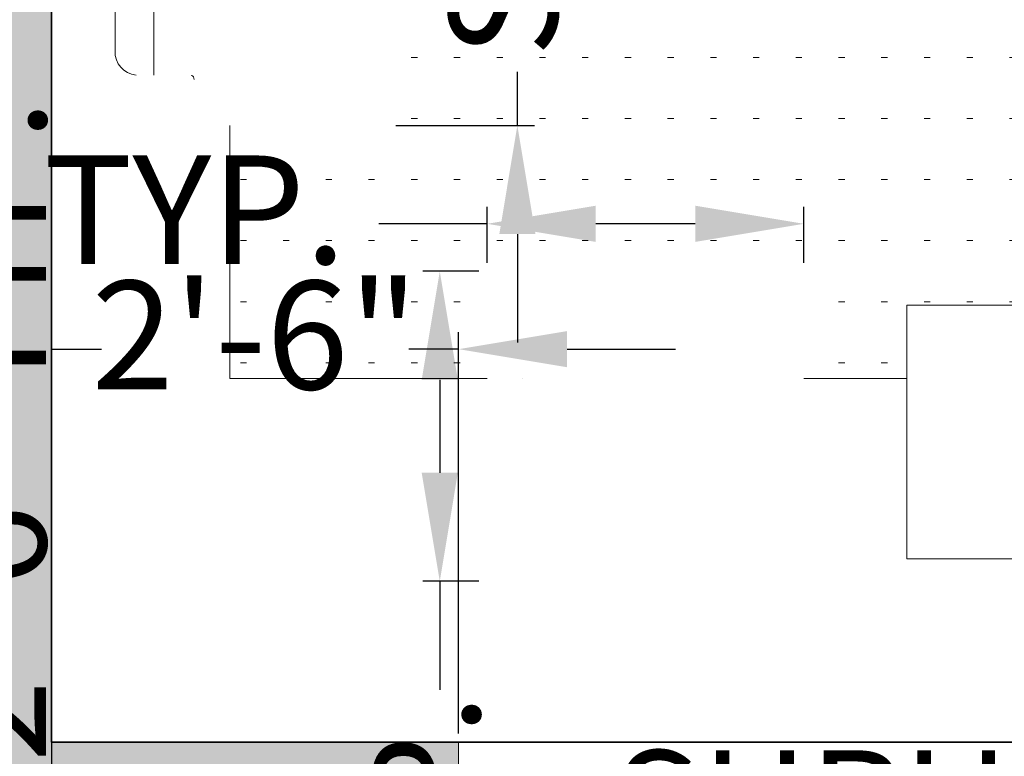
# Model space of a CAD drawing. Units: inches. Extents: x 2408 to 5087, y 2429 to 5085.
# Tile 4 of 12: x 2491 to 2564, y 2622 to 2676. Entities that reach past the tile are written whole.
import ezdxf

# ---------------------------------------------------------------- set-up
doc = ezdxf.new("R2010")
doc.units = ezdxf.units.IN
for name, color, linetype, lineweight in [('A-ANNO-DIMS', 2, 'Continuous', 18), ('A-FLOR-PATT', 8, 'Continuous', 13), ('A-FURN', 72, 'Continuous', 18), ('A-GLAZ', 4, 'Continuous', 18), ('A-WALL', 7, 'Continuous', 35), ('A-WALL-PATT', 252, 'Continuous', 13)]:
    doc.layers.add(name, color=color, linetype=linetype, lineweight=lineweight)
doc.styles.get("Standard").update_dxf_attribs({"font": 'arial.ttf'})
doc.dimstyles.new('ISO-25', dxfattribs={"dimtxt": 8, "dimasz": 8, "dimexe": 1.25, "dimexo": 0.625, "dimtad": 0, "dimdec": 1, "dimlunit": 4, "dimtxsty": 'Standard', "dimcen": 2.5, "dimadec": 0, "dimazin": 0, "dimtfac": 1, "dimtdec": 1, "dimtmove": 0, "dimatfit": 3, "dimfxl": 1, "dimarcsym": 0})

# ---------------------------------------------------------------- blocks, each defined once
blk = doc.blocks.new('Clinicians and patient chairs 9_dwgmodels.com')
at = {"color": 0}
for points in [[(-907.9, 0, 0, 0, 0), (-959.6, -11.1, 4.62, 4.62, 0)], [(907.9, 0, 0, 0, 0), (-907.9, 0, 4.62, 4.62, 0)], [(959.6, -11.1, 0, 0, 0), (907.9, 0, 4.62, 4.62, 0)], [(-959.6, -11.1, 0, 0, 0), (-994.7, -35.9, 4.62, 4.62, 0)], [(994.7, -35.9, 0, 0, 0), (959.6, -11.1, 4.62, 4.62, 0)], [(-994.7, -35.9, 0, 0, 0), (-1015.6, -68.3, 4.62, 4.62, 0)], [(1015.6, -68.3, 0, 0, 0), (994.7, -35.9, 4.62, 4.62, 0)], [(-1015.6, -68.3, 0, 0, 0), (-1025.5, -106.3, 4.62, 4.62, 0)], [(1025.5, -106.3, 0, 0, 0), (1015.6, -68.3, 4.62, 4.62, 0)], [(-1025.5, -106.3, 0, 0, 0), (-1025.5, -779.5, 4.62, 4.62, 0)], [(1025.5, -779.5, 0, 0, 0), (1025.5, -106.3, 4.62, 4.62, 0)], [(1025.5, -779.5, 0, 0, 0), (1025.5, -117.3, 4.62, 4.62, 0)], [(-313.4, -149.9, 0, 0, 0), (-318.1, -149.9, 4.62, 4.62, 0)], [(-314.5, -150.4, 0, 0, 0), (-315.7, -159.3, 4.62, 4.62, 0)], [(-315.7, -159.3, 0, 0, 0), (-315.7, -777.3, 4.62, 4.62, 0)], [(-309.5, -148.3, 0, 0, 0), (-314.5, -150.4, 4.62, 4.62, 0)], [(-308, -148.3, 0, 0, 0), (-309.5, -148.3, 4.62, 4.62, 0)], [(-307.5, -148.3, 0, 0, 0), (-308, -148.3, 4.62, 4.62, 0)], [(242.9, -148.3, 0, 0, 0), (-307.5, -148.3, 4.62, 4.62, 0)], [(242.9, -148.3, 0, 0, 0), (296, -148.3, 4.62, 4.62, 0)], [(296, -148.3, 0, 0, 0), (307.5, -148.3, 4.62, 4.62, 0)], [(308, -148.3, 0, 0, 0), (307.5, -148.3, 4.62, 4.62, 0)], [(309.5, -148.3, 0, 0, 0), (308, -148.3, 4.62, 4.62, 0)], [(309.5, -148.3, 0, 0, 0), (314.5, -150.4, 4.62, 4.62, 0)], [(849.5, -149.9, 0, 0, 0), (313.4, -149.9, 4.62, 4.62, 0)], [(314.5, -150.4, 0, 0, 0), (315.7, -159.3, 4.62, 4.62, 0)], [(315.7, -159.3, 0, 0, 0), (315.7, -777.3, 4.62, 4.62, 0)], [(315.7, -161.8, 0, 0, 0), (315.7, -777.3, 4.62, 4.62, 0)], [(-906.6, -285, 0, 0, 0), (-906.4, -198.1, 4.62, 4.62, 0)], [(906.9, -327, 0, 0, 0), (906.4, -199.7, 4.62, 4.62, 0)], [(-906.6, -285, 0, 0, 0), (-906.8, -305.4, 4.62, 4.62, 0)], [(-906.8, -305.4, 0, 0, 0), (-906.9, -324.5, 4.62, 4.62, 0)], [(-906.9, -324.5, 0, 0, 0), (-906.9, -329.8, 4.62, 4.62, 0)], [(906.9, -327, 0, 0, 0), (906.9, -329.9, 4.62, 4.62, 0)], [(-1023, -329.7, 0, 0, 0), (-1019.2, -332.9, 4.62, 4.62, 0)], [(-1019.8, -340.2, 0, 0, 0), (-1023, -348.6, 4.62, 4.62, 0)], [(-1010.3, -335.9, 0, 0, 0), (-1019.8, -340.2, 4.62, 4.62, 0)], [(-1019.2, -332.9, 0, 0, 0), (-1019, -333, 4.62, 4.62, 0)], [(-1019, -333, 0, 0, 0), (-1018.9, -333.1, 4.62, 4.62, 0)], [(-1013.9, -334.2, 0, 0, 0), (-1018.9, -333.1, 4.62, 4.62, 0)], [(-1013.9, -334.2, 0, 0, 0), (-964.4, -335.7, 4.62, 4.62, 0)], [(-917.1, -337, 0, 0, 0), (-1010.3, -335.9, 4.62, 4.62, 0)], [(-964.4, -335.7, 0, 0, 0), (-927.1, -336.8, 4.62, 4.62, 0)], [(964.4, -335.7, 0, 0, 0), (914.9, -337.2, 4.62, 4.62, 0)], [(917.1, -339.4, 0, 0, 0), (1010.3, -338.4, 4.62, 4.62, 0)], [(1013.9, -334.2, 0, 0, 0), (964.4, -335.7, 4.62, 4.62, 0)], [(1010.3, -338.4, 0, 0, 0), (1019.8, -342.7, 4.62, 4.62, 0)], [(1013.9, -334.2, 0, 0, 0), (1018.9, -333.1, 4.62, 4.62, 0)], [(1018.9, -333.1, 0, 0, 0), (1019, -333, 4.62, 4.62, 0)], [(1019.2, -332.9, 0, 0, 0), (1019, -333, 4.62, 4.62, 0)], [(1023, -329.7, 0, 0, 0), (1019.2, -332.9, 4.62, 4.62, 0)], [(1019.8, -342.7, 0, 0, 0), (1023, -351.1, 4.62, 4.62, 0)], [(1023, -351.1, 0, 0, 0), (1022.6, -779.8, 4.62, 4.62, 0)], [(-1025.5, -779.5, 0, 0, 0), (-1022.2, -788.7, 4.62, 4.62, 0)], [(-1022.2, -788.7, 0, 0, 0), (-1021.6, -789.8, 4.62, 4.62, 0)], [(-1021.6, -789.8, 0, 0, 0), (-1020.6, -790.5, 4.62, 4.62, 0)], [(-1020.6, -790.5, 0, 0, 0), (-1013.6, -793.7, 4.62, 4.62, 0)], [(-1013.6, -793.7, 0, 0, 0), (1013.6, -793.7, 4.62, 4.62, 0)], [(1019.8, -788.8, 0, 0, 0), (1013.1, -793.7, 4.62, 4.62, 0)], [(1013.6, -793.7, 0, 0, 0), (1020.6, -790.5, 4.62, 4.62, 0)], [(1022.6, -779.8, 0, 0, 0), (1019.8, -788.8, 4.62, 4.62, 0)], [(1020.6, -790.5, 0, 0, 0), (1021.6, -789.8, 4.62, 4.62, 0)], [(1022.2, -788.7, 0, 0, 0), (1021.6, -789.8, 4.62, 4.62, 0)], [(1022.2, -788.7, 0, 0, 0), (1025.5, -779.5, 4.62, 4.62, 0)]]:
    blk.add_lwpolyline(points, format="xyseb", dxfattribs=at)
for points in [[(-849.5, -149.9), (-318.1, -149.9)], [(-906.5, -241.5), (906.5, -242.3)]]:
    blk.add_lwpolyline(points, dxfattribs=at)
for centre, radius, start, end in [((-851.7, -204.8), 54.9, 87.6679, 174.7256), ((851.7, -204.8), 54.9, 5.2744, 92.3321), ((-916.6, -326.8), 10.2, 267.5454, 342.4057), ((916.9, -329.4), 10, 182.6094, 270.795), ((-337, -773.8), 21.5, 292.115, 350.6304), ((-294.5, -773.8), 21.5, 189.3696, 247.885), ((294.5, -773.8), 21.5, 292.115, 350.6304), ((336.9, -773.8), 21.5, 189.3696, 247.885)]:
    blk.add_arc(centre, radius, start, end, dxfattribs=at)
blk.add_point((0, -793.7), dxfattribs=at)
blk = doc.blocks.new('Clinicians and patient chairs 25_dwgmodels.com')
at = {"color": 0}
for points in [[(-289.5, -1.5, 0, 0, 0), (-290.1, -3.2, 4.37, 4.37, 0)], [(-287.1, -0.3, 0, 0, 0), (-289.5, -1.5, 4.37, 4.37, 0)], [(-287.1, -0.3, 0, 0, 0), (-265.1, -0.9, 4.37, 4.37, 0)], [(-265.1, -0.9, 0, 0, 0), (-198.5, -0.4, 4.37, 4.37, 0)], [(-198.5, -0.4, 0, 0, 0), (-92.3, -0.3, 4.37, 4.37, 0)], [(-92.3, -0.3, 0, 0, 0), (0, 0, 4.37, 4.37, 0)], [(92.3, -0.3, 0, 0, 0), (0, 0, 4.37, 4.37, 0)], [(198.5, -0.4, 0, 0, 0), (92.3, -0.3, 4.37, 4.37, 0)], [(265.7, -0.9, 0, 0, 0), (198.5, -0.4, 4.37, 4.37, 0)], [(287.7, -0.3, 0, 0, 0), (265.7, -0.9, 4.37, 4.37, 0)], [(287.7, -0.3, 0, 0, 0), (290.1, -1.5, 4.37, 4.37, 0)], [(290.1, -1.5, 0, 0, 0), (290.7, -3.2, 4.37, 4.37, 0)], [(-371.8, -16.6, 0, 0, 0), (-369.1, -9.1, 4.37, 4.37, 0)], [(-371.8, -16.5, 0, 0, 0), (-369.8, -11, 4.37, 4.37, 0)], [(-371.8, -16.6, 0, 0, 0), (-371.8, -705.5, 4.37, 4.37, 0)], [(-371.8, -16.6, 0, 0, 0), (-371.8, -705.5, 4.37, 4.37, 0)], [(-369.8, -8.3, 0, 0, 0), (-369.7, -10.5, 4.37, 4.37, 0)], [(-369.8, -8.3, 0, 0, 0), (-369.8, -9.6, 4.37, 4.37, 0)], [(-369.8, -8.3, 0, 0, 0), (-367.7, -8.5, 4.37, 4.37, 0)], [(-369.8, -11, 0, 0, 0), (-369.8, -11, 4.37, 4.37, 0)], [(-369.8, -11, 0, 0, 0), (-369.8, -11, 4.37, 4.37, 0)], [(-369.8, -11, 0, 0, 0), (-369.8, -11, 4.37, 4.37, 0)], [(-369.7, -10.5, 0, 0, 0), (-369.6, -10.6, 4.37, 4.37, 0)], [(-369.1, -9.1, 0, 0, 0), (-361.2, -6.5, 4.37, 4.37, 0)], [(-367.7, -8.5, 0, 0, 0), (-367.6, -8.6, 4.37, 4.37, 0)], [(-367.7, -8.5, 0, 0, 0), (-367.6, -8.6, 4.37, 4.37, 0)], [(-361.2, -6.5, 0, 0, 0), (-367.2, -8.4, 4.37, 4.37, 0)], [(-367.2, -8.4, 0, 0, 0), (-367.2, -8.4, 4.37, 4.37, 0)], [(-367.2, -8.5, 0, 0, 0), (-367.2, -8.4, 4.37, 4.37, 0)], [(-299.5, -6.5, 0, 0, 0), (-361.2, -6.5, 4.37, 4.37, 0)], [(-299.5, -6.5, 0, 0, 0), (-294.7, -8, 4.37, 4.37, 0)], [(-299.5, -6.5, 0, 0, 0), (-294.7, -8.1, 4.37, 4.37, 0)], [(-294.7, -6.7, 0, 0, 0), (-291.8, -2.6, 4.37, 4.37, 0)], [(-294.8, -31.9, 0, 0, 0), (-294.7, -6.7, 4.37, 4.37, 0)], [(-294.7, -29.9, 0, 0, 0), (-294.5, -13.6, 4.37, 4.37, 0)], [(-291.8, -2.6, 0, 0, 0), (-290.1, -3.2, 4.37, 4.37, 0)], [(-289.7, -10.8, 0, 0, 0), (-290.1, -3.2, 4.37, 4.37, 0)], [(-290, -30, 0, 0, 0), (-289.7, -10.8, 4.37, 4.37, 0)], [(290.3, -10.8, 0, 0, 0), (290.7, -3.2, 4.37, 4.37, 0)], [(290.7, -30, 0, 0, 0), (290.3, -10.8, 4.37, 4.37, 0)], [(292.4, -2.6, 0, 0, 0), (290.7, -3.2, 4.37, 4.37, 0)], [(295.4, -6.7, 0, 0, 0), (292.4, -2.6, 4.37, 4.37, 0)], [(295.4, -29.9, 0, 0, 0), (295.1, -13.6, 4.37, 4.37, 0)], [(299.5, -6.5, 0, 0, 0), (295.4, -7.9, 4.37, 4.37, 0)], [(299.5, -6.5, 0, 0, 0), (295.4, -7.8, 4.37, 4.37, 0)], [(295.4, -31.9, 0, 0, 0), (295.4, -6.7, 4.37, 4.37, 0)], [(299.5, -6.5, 0, 0, 0), (361.2, -6.5, 4.37, 4.37, 0)], [(369.1, -9.1, 0, 0, 0), (361.2, -6.5, 4.37, 4.37, 0)], [(369.1, -9.1, 0, 0, 0), (361.2, -6.5, 4.37, 4.37, 0)], [(361.2, -6.6, 0, 0, 0), (367.2, -8.4, 4.37, 4.37, 0)], [(367.2, -8.4, 0, 0, 0), (367.2, -8.4, 4.37, 4.37, 0)], [(367.2, -8.5, 0, 0, 0), (367.2, -8.4, 4.37, 4.37, 0)], [(367.7, -8.5, 0, 0, 0), (367.6, -8.6, 4.37, 4.37, 0)], [(367.7, -8.5, 0, 0, 0), (367.6, -8.6, 4.37, 4.37, 0)], [(369.8, -8.3, 0, 0, 0), (367.7, -8.5, 4.37, 4.37, 0)], [(371.8, -16.6, 0, 0, 0), (369.1, -9.1, 4.37, 4.37, 0)], [(369.4, -10, 0, 0, 0), (369.4, -10, 4.37, 4.37, 0)], [(369.7, -10.5, 0, 0, 0), (369.6, -10.6, 4.37, 4.37, 0)], [(369.8, -8.3, 0, 0, 0), (369.7, -10.5, 4.37, 4.37, 0)], [(369.8, -8.3, 0, 0, 0), (369.8, -9.6, 4.37, 4.37, 0)], [(371.8, -16.5, 0, 0, 0), (369.8, -11, 4.37, 4.37, 0)], [(369.8, -11, 0, 0, 0), (369.8, -11, 4.37, 4.37, 0)], [(369.8, -11, 0, 0, 0), (369.8, -11, 4.37, 4.37, 0)], [(369.8, -11, 0, 0, 0), (369.8, -11, 4.37, 4.37, 0)], [(371.8, -16.6, 0, 0, 0), (371.8, -705.5, 4.37, 4.37, 0)], [(-371.8, -44.1, 0, 0, 0), (-371.8, -361, 4.37, 4.37, 0)], [(-294.8, -48.3, 0, 0, 0), (-294.8, -31.9, 4.37, 4.37, 0)], [(-294.8, -48.3, 0, 0, 0), (-294.7, -60.2, 4.37, 4.37, 0)], [(-294.7, -29.9, 0, 0, 0), (-294.8, -31.9, 4.37, 4.37, 0)], [(-290.1, -51.3, 0, 0, 0), (-290, -30, 4.37, 4.37, 0)], [(290.7, -51.3, 0, 0, 0), (290.7, -30, 4.37, 4.37, 0)], [(295.4, -29.9, 0, 0, 0), (295.4, -31.9, 4.37, 4.37, 0)], [(295.4, -31.9, 0, 0, 0), (295.4, -48.3, 4.37, 4.37, 0)], [(295.4, -60.2, 0, 0, 0), (295.4, -48.3, 4.37, 4.37, 0)], [(371.8, -44.1, 0, 0, 0), (371.8, -361, 4.37, 4.37, 0)], [(-294.7, -60.2, 0, 0, 0), (-294.7, -69.9, 4.37, 4.37, 0)], [(-294.7, -69.9, 0, 0, 0), (-294.7, -86.3, 4.37, 4.37, 0)], [(-290, -64.7, 0, 0, 0), (-290.1, -51.3, 4.37, 4.37, 0)], [(-290, -64.7, 0, 0, 0), (-290, -74.5, 4.37, 4.37, 0)], [(-284.2, -72.8, 0, 0, 0), (-262.5, -66.3, 4.37, 4.37, 0)], [(-283.3, -75.9, 0, 0, 0), (-262, -69.5, 4.37, 4.37, 0)], [(-280.9, -71.1, 0, 0, 0), (-282.2, -72.2, 4.37, 4.37, 0)], [(-276.4, -68.7, 0, 0, 0), (-280.9, -71.1, 4.37, 4.37, 0)], [(-276.4, -68.7, 0, 0, 0), (-257.9, -63.2, 4.37, 4.37, 0)], [(-262.5, -66.3, 0, 0, 0), (-233.5, -62.8, 4.37, 4.37, 0)], [(-262, -69.5, 0, 0, 0), (-233.2, -66.1, 4.37, 4.37, 0)], [(-257.9, -63.2, 0, 0, 0), (-233.1, -60.2, 4.37, 4.37, 0)], [(-233.5, -62.8, 0, 0, 0), (-96.6, -62.8, 4.37, 4.37, 0)], [(-96.6, -66, 0, 0, 0), (-233.2, -66.1, 4.37, 4.37, 0)], [(-233.1, -60.2, 0, 0, 0), (-96.5, -60.1, 4.37, 4.37, 0)], [(126.5, -62.8, 0, 0, 0), (-96.6, -62.8, 4.37, 4.37, 0)], [(126.5, -66, 0, 0, 0), (-96.6, -66, 4.37, 4.37, 0)], [(126.4, -60.1, 0, 0, 0), (-96.5, -60.1, 4.37, 4.37, 0)], [(233.6, -60.2, 0, 0, 0), (126.4, -60.1, 4.37, 4.37, 0)], [(234, -62.8, 0, 0, 0), (126.5, -62.8, 4.37, 4.37, 0)], [(126.5, -66, 0, 0, 0), (233.8, -66.1, 4.37, 4.37, 0)], [(258.5, -63.2, 0, 0, 0), (233.6, -60.2, 4.37, 4.37, 0)], [(262.5, -69.5, 0, 0, 0), (233.8, -66.1, 4.37, 4.37, 0)], [(234, -62.8, 0, 0, 0), (263.1, -66.3, 4.37, 4.37, 0)], [(277, -68.7, 0, 0, 0), (258.5, -63.2, 4.37, 4.37, 0)], [(262.5, -69.5, 0, 0, 0), (283.8, -75.9, 4.37, 4.37, 0)], [(284.7, -72.8, 0, 0, 0), (263.1, -66.3, 4.37, 4.37, 0)], [(277, -68.7, 0, 0, 0), (281.4, -71.1, 4.37, 4.37, 0)], [(281.4, -71.1, 0, 0, 0), (282.8, -72.2, 4.37, 4.37, 0)], [(290.7, -64.7, 0, 0, 0), (290.7, -51.3, 4.37, 4.37, 0)], [(290.6, -74.5, 0, 0, 0), (290.7, -64.7, 4.37, 4.37, 0)], [(295.4, -60.2, 0, 0, 0), (295.4, -69.9, 4.37, 4.37, 0)], [(295.4, -69.9, 0, 0, 0), (295.3, -86.3, 4.37, 4.37, 0)], [(-293, -92.7, 0, 0, 0), (-295.9, -118.4, 4.37, 4.37, 0)], [(-294.7, -86.3, 0, 0, 0), (-294.7, -87.6, 4.37, 4.37, 0)], [(-294.7, -87.6, 0, 0, 0), (-294.7, -87.7, 4.37, 4.37, 0)], [(-294.5, -88.2, 0, 0, 0), (-294.7, -87.7, 4.37, 4.37, 0)], [(-292.8, -91.5, 0, 0, 0), (-294.5, -88.2, 4.37, 4.37, 0)], [(-293, -92.7, 0, 0, 0), (-291.6, -83.8, 4.37, 4.37, 0)], [(-291.8, -79.4, 0, 0, 0), (-284.2, -72.8, 4.37, 4.37, 0)], [(-291.8, -79.4, 0, 0, 0), (-291.8, -84.9, 4.37, 4.37, 0)], [(-291.6, -83.8, 0, 0, 0), (-290.8, -82.4, 4.37, 4.37, 0)], [(-283.3, -75.9, 0, 0, 0), (-290.8, -82.4, 4.37, 4.37, 0)], [(-290, -74.5, 0, 0, 0), (-290, -77.9, 4.37, 4.37, 0)], [(283.8, -75.9, 0, 0, 0), (289.6, -80.9, 4.37, 4.37, 0)], [(284.7, -72.8, 0, 0, 0), (291.2, -78.5, 4.37, 4.37, 0)], [(289.8, -81.8, 0, 0, 0), (289.6, -80.9, 4.37, 4.37, 0)], [(289.8, -81.8, 0, 0, 0), (291.4, -92.3, 4.37, 4.37, 0)], [(290.6, -74.5, 0, 0, 0), (290.7, -78, 4.37, 4.37, 0)], [(292.4, -98.2, 0, 0, 0), (291.2, -78.5, 4.37, 4.37, 0)], [(294.4, -118.8, 0, 0, 0), (291.4, -92.3, 4.37, 4.37, 0)], [(292.1, -93.2, 0, 0, 0), (292.6, -93.1, 4.37, 4.37, 0)], [(292.8, -92.7, 0, 0, 0), (292.6, -93.1, 4.37, 4.37, 0)], [(292.8, -92.7, 0, 0, 0), (294.5, -89.3, 4.37, 4.37, 0)], [(294.5, -89.3, 0, 0, 0), (294.9, -88.5, 4.37, 4.37, 0)], [(294.9, -88.5, 0, 0, 0), (295.3, -87.6, 4.37, 4.37, 0)], [(295.3, -86.3, 0, 0, 0), (295.3, -87.8, 4.37, 4.37, 0)], [(292.3, -100.4, 0, 0, 0), (292.4, -100.3, 4.37, 4.37, 0)], [(292.4, -100.2, 0, 0, 0), (292.4, -98.2, 4.37, 4.37, 0)], [(-295.9, -118.4, 0, 0, 0), (-295.9, -139.7, 4.37, 4.37, 0)], [(-295.9, -139.7, 0, 0, 0), (-295.9, -144.1, 4.37, 4.37, 0)], [(294.4, -118.8, 0, 0, 0), (296.4, -139.7, 4.37, 4.37, 0)], [(296.4, -139.7, 0, 0, 0), (296.4, -144.7, 4.37, 4.37, 0)], [(-295.6, -147.4, 0, 0, 0), (-295.9, -144.1, 4.37, 4.37, 0)], [(-295.6, -147.4, 0, 0, 0), (-294.9, -155.8, 4.37, 4.37, 0)], [(-294.9, -155.8, 0, 0, 0), (-294, -165.2, 4.37, 4.37, 0)], [(-292.1, -160, 0, 0, 0), (-291, -157.5, 4.37, 4.37, 0)], [(-292.1, -182.8, 0, 0, 0), (-292.1, -160, 4.37, 4.37, 0)], [(-283.4, -148.6, 0, 0, 0), (-291, -157.5, 4.37, 4.37, 0)], [(-289, -161.1, 0, 0, 0), (-289.1, -183.8, 4.37, 4.37, 0)], [(-288.7, -160.4, 0, 0, 0), (-289, -161.1, 4.37, 4.37, 0)], [(-283.4, -148.6, 0, 0, 0), (-262.3, -142.9, 4.37, 4.37, 0)], [(-261.4, -146.5, 0, 0, 0), (-282, -152.1, 4.37, 4.37, 0)], [(-261.8, -142.8, 0, 0, 0), (-262.3, -142.9, 4.37, 4.37, 0)], [(-261.4, -146.5, 0, 0, 0), (-233.4, -145.3, 4.37, 4.37, 0)], [(-233.4, -145.3, 0, 0, 0), (-96.7, -145.6, 4.37, 4.37, 0)], [(-96.7, -145.6, 0, 0, 0), (126.7, -145.6, 4.37, 4.37, 0)], [(233.9, -145.3, 0, 0, 0), (126.7, -145.6, 4.37, 4.37, 0)], [(261.9, -146.5, 0, 0, 0), (233.9, -145.3, 4.37, 4.37, 0)], [(261.9, -146.5, 0, 0, 0), (282.5, -152.1, 4.37, 4.37, 0)], [(262.4, -142.8, 0, 0, 0), (262.8, -142.9, 4.37, 4.37, 0)], [(283.9, -148.6, 0, 0, 0), (262.8, -142.9, 4.37, 4.37, 0)], [(283.9, -148.6, 0, 0, 0), (291.5, -157.5, 4.37, 4.37, 0)], [(289.2, -160.4, 0, 0, 0), (289.6, -161.1, 4.37, 4.37, 0)], [(289.6, -161.1, 0, 0, 0), (289.6, -183.8, 4.37, 4.37, 0)], [(292.6, -160, 0, 0, 0), (291.5, -157.5, 4.37, 4.37, 0)], [(292.6, -160, 0, 0, 0), (292.7, -182.8, 4.37, 4.37, 0)], [(294.1, -170, 0, 0, 0), (294.9, -162, 4.37, 4.37, 0)], [(294.9, -162, 0, 0, 0), (296.2, -147, 4.37, 4.37, 0)], [(296.2, -147, 0, 0, 0), (296.4, -144.1, 4.37, 4.37, 0)], [(-294, -165.2, 0, 0, 0), (-293.2, -174.7, 4.37, 4.37, 0)], [(-292.1, -183.2, 0, 0, 0), (-293.2, -174.7, 4.37, 4.37, 0)], [(-292.1, -182.8, 0, 0, 0), (-292.1, -189.8, 4.37, 4.37, 0)], [(-289.1, -192.9, 0, 0, 0), (-289.1, -183.8, 4.37, 4.37, 0)], [(289.6, -183.8, 0, 0, 0), (289.6, -191.3, 4.37, 4.37, 0)], [(292.7, -183.1, 0, 0, 0), (293.7, -174.6, 4.37, 4.37, 0)], [(292.7, -182.8, 0, 0, 0), (292.7, -189.8, 4.37, 4.37, 0)], [(294, -171.7, 0, 0, 0), (293.7, -174.6, 4.37, 4.37, 0)], [(294.1, -170, 0, 0, 0), (294, -171.7, 4.37, 4.37, 0)], [(-291, -191.1, 0, 0, 0), (-292.1, -190.5, 4.37, 4.37, 0)], [(-290.4, -191.5, 0, 0, 0), (-291, -191.1, 4.37, 4.37, 0)], [(-290, -191.9, 0, 0, 0), (-290.4, -191.5, 4.37, 4.37, 0)], [(-290, -191.9, 0, 0, 0), (-289.4, -192.4, 4.37, 4.37, 0)], [(-289.1, -192.4, 0, 0, 0), (-289.4, -192.4, 4.37, 4.37, 0)], [(-288.9, -193.4, 0, 0, 0), (-289.1, -192.9, 4.37, 4.37, 0)], [(-288.9, -193.4, 0, 0, 0), (-288.9, -193.4, 4.37, 4.37, 0)], [(-288.9, -194.1, 0, 0, 0), (-288.9, -686.6, 4.37, 4.37, 0)], [(-288.9, -197.7, 0, 0, 0), (-288.9, -361, 4.37, 4.37, 0)], [(-288.9, -197.7, 0, 0, 0), (-288.9, -686.6, 4.37, 4.37, 0)], [(289.5, -193, 0, 0, 0), (288.9, -194.6, 4.37, 4.37, 0)], [(288.9, -194.1, 0, 0, 0), (288.9, -686.6, 4.37, 4.37, 0)], [(288.9, -199.4, 0, 0, 0), (288.9, -361, 4.37, 4.37, 0)], [(289.5, -193, 0, 0, 0), (289.6, -192.6, 4.37, 4.37, 0)], [(289.8, -192.1, 0, 0, 0), (289.6, -192, 4.37, 4.37, 0)], [(289.8, -192.1, 0, 0, 0), (290, -192.1, 4.37, 4.37, 0)], [(290.4, -191.7, 0, 0, 0), (290, -192.1, 4.37, 4.37, 0)], [(290.5, -191.6, 0, 0, 0), (291, -191.2, 4.37, 4.37, 0)], [(290.5, -191.6, 0, 0, 0), (290.4, -191.7, 4.37, 4.37, 0)], [(291, -191.2, 0, 0, 0), (292.7, -190.4, 4.37, 4.37, 0)], [(-288.3, -246.3, 0, 0, 0), (-288.9, -245.1, 4.37, 4.37, 0)], [(-286.9, -248.4, 0, 0, 0), (-288.9, -247.9, 4.37, 4.37, 0)], [(-288.3, -246.3, 0, 0, 0), (-286, -249.9, 4.37, 4.37, 0)], [(-281.3, -252.3, 0, 0, 0), (-286, -249.9, 4.37, 4.37, 0)], [(-281.3, -252.3, 0, 0, 0), (-276, -253.6, 4.37, 4.37, 0)], [(-276, -253.6, 0, 0, 0), (-230.3, -254.3, 4.37, 4.37, 0)], [(-230.3, -254.3, 0, 0, 0), (-94.3, -254.3, 4.37, 4.37, 0)], [(124.3, -254.3, 0, 0, 0), (-94.3, -254.3, 4.37, 4.37, 0)], [(230.8, -254.3, 0, 0, 0), (124.3, -254.3, 4.37, 4.37, 0)], [(276.5, -253.6, 0, 0, 0), (230.8, -254.3, 4.37, 4.37, 0)], [(281.8, -252.3, 0, 0, 0), (276.5, -253.6, 4.37, 4.37, 0)], [(281.8, -252.3, 0, 0, 0), (286.5, -249.9, 4.37, 4.37, 0)], [(286.5, -249.9, 0, 0, 0), (288.9, -246.3, 4.37, 4.37, 0)], [(287.5, -248.4, 0, 0, 0), (288.9, -248, 4.37, 4.37, 0)], [(288.9, -246.3, 0, 0, 0), (288.9, -246.2, 4.37, 4.37, 0)], [(-371.8, -705.5, 0, 0, 0), (-371.8, -361, 4.37, 4.37, 0)], [(-288.9, -705.5, 0, 0, 0), (-288.9, -361, 4.37, 4.37, 0)], [(288.9, -686.6, 0, 0, 0), (288.9, -361, 4.37, 4.37, 0)], [(371.8, -705.5, 0, 0, 0), (371.8, -361, 4.37, 4.37, 0)], [(-288.9, -686.9, 0, 0, 0), (-288.9, -705.5, 4.37, 4.37, 0)], [(-288.9, -686.9, 0, 0, 0), (-288.9, -705.5, 4.37, 4.37, 0)], [(288.9, -686.9, 0, 0, 0), (288.9, -705.5, 4.37, 4.37, 0)], [(288.9, -705.5, 0, 0, 0), (288.9, -686.9, 4.37, 4.37, 0)], [(-371.8, -705.5, 0, 0, 0), (-369.8, -711.1, 4.37, 4.37, 0)], [(-371.8, -705.5, 0, 0, 0), (-369.1, -713, 4.37, 4.37, 0)], [(-369.8, -711.1, 0, 0, 0), (-369.8, -711.1, 4.37, 4.37, 0)], [(-369.8, -711.1, 0, 0, 0), (-369.8, -711.1, 4.37, 4.37, 0)], [(-369.8, -713.8, 0, 0, 0), (-369.7, -711.6, 4.37, 4.37, 0)], [(-369.8, -713.8, 0, 0, 0), (-367.7, -713.6, 4.37, 4.37, 0)], [(-369.8, -713.8, 0, 0, 0), (-368.6, -713.7, 4.37, 4.37, 0)], [(-369.7, -711.6, 0, 0, 0), (-369.7, -711.5, 4.37, 4.37, 0)], [(-369.3, -712.5, 0, 0, 0), (-369.2, -712.7, 4.37, 4.37, 0)], [(-369.2, -712.7, 0, 0, 0), (-369.2, -712.8, 4.37, 4.37, 0)], [(-369.1, -713, 0, 0, 0), (-361.2, -715.5, 4.37, 4.37, 0)], [(-367.7, -713.6, 0, 0, 0), (-367.6, -713.5, 4.37, 4.37, 0)], [(-367.7, -713.6, 0, 0, 0), (-367.6, -713.5, 4.37, 4.37, 0)], [(-367.2, -713.7, 0, 0, 0), (-367.2, -713.6, 4.37, 4.37, 0)], [(-367.2, -713.6, 0, 0, 0), (-367.2, -713.6, 4.37, 4.37, 0)], [(-361.2, -715.5, 0, 0, 0), (-367.2, -713.7, 4.37, 4.37, 0)], [(-361.2, -715.5, 0, 0, 0), (-299.5, -715.5, 4.37, 4.37, 0)], [(-299.5, -715.5, 0, 0, 0), (-361.2, -715.5, 4.37, 4.37, 0)], [(-299.5, -715.5, 0, 0, 0), (-291.6, -713, 4.37, 4.37, 0)], [(-299.5, -715.5, 0, 0, 0), (-293.5, -713.7, 4.37, 4.37, 0)], [(-294.3, -713.9, 0, 0, 0), (-291.6, -721.7, 4.37, 4.37, 0)], [(-293, -713.6, 0, 0, 0), (-293.1, -713.5, 4.37, 4.37, 0)], [(-290.8, -713.8, 0, 0, 0), (-293, -713.6, 4.37, 4.37, 0)], [(-288.9, -705.5, 0, 0, 0), (-291.6, -713, 4.37, 4.37, 0)], [(-288.9, -705.5, 0, 0, 0), (-291.6, -713, 4.37, 4.37, 0)], [(-291.5, -713.7, 0, 0, 0), (-291.5, -715.5, 4.37, 4.37, 0)], [(-291.4, -721.7, 0, 0, 0), (-291.5, -715.5, 4.37, 4.37, 0)], [(-290.9, -711.6, 0, 0, 0), (-291, -711.5, 4.37, 4.37, 0)], [(-288.9, -705.5, 0, 0, 0), (-290.9, -711.1, 4.37, 4.37, 0)], [(-290.9, -713.8, 0, 0, 0), (-290.9, -711.6, 4.37, 4.37, 0)], [(-290.8, -713.8, 0, 0, 0), (-290.9, -712.4, 4.37, 4.37, 0)], [(288.9, -705.5, 0, 0, 0), (291.6, -713, 4.37, 4.37, 0)], [(288.9, -705.5, 0, 0, 0), (291.6, -713, 4.37, 4.37, 0)], [(288.9, -705.5, 0, 0, 0), (290.9, -711.1, 4.37, 4.37, 0)], [(290.9, -713.8, 0, 0, 0), (290.9, -711.6, 4.37, 4.37, 0)], [(290.8, -713.8, 0, 0, 0), (290.9, -712.4, 4.37, 4.37, 0)], [(290.8, -713.8, 0, 0, 0), (293, -713.6, 4.37, 4.37, 0)], [(290.9, -711.6, 0, 0, 0), (291, -711.5, 4.37, 4.37, 0)], [(291.4, -721.7, 0, 0, 0), (291.5, -715.5, 4.37, 4.37, 0)], [(291.5, -713.7, 0, 0, 0), (291.5, -715.5, 4.37, 4.37, 0)], [(299.5, -715.5, 0, 0, 0), (291.6, -713, 4.37, 4.37, 0)], [(294.3, -713.9, 0, 0, 0), (291.6, -721.7, 4.37, 4.37, 0)], [(293, -713.6, 0, 0, 0), (293.1, -713.5, 4.37, 4.37, 0)], [(299.5, -715.5, 0, 0, 0), (293.5, -713.7, 4.37, 4.37, 0)], [(299.5, -715.5, 0, 0, 0), (361.2, -715.5, 4.37, 4.37, 0)], [(299.5, -715.5, 0, 0, 0), (361.2, -715.5, 4.37, 4.37, 0)], [(299.5, -715.5, 0, 0, 0), (361.2, -715.5, 4.37, 4.37, 0)], [(361.2, -715.5, 0, 0, 0), (299.5, -715.5, 4.37, 4.37, 0)], [(369.1, -713, 0, 0, 0), (361.2, -715.5, 4.37, 4.37, 0)], [(369.1, -713, 0, 0, 0), (361.2, -715.5, 4.37, 4.37, 0)], [(361.2, -715.5, 0, 0, 0), (367.2, -713.7, 4.37, 4.37, 0)], [(367.2, -713.6, 0, 0, 0), (367.2, -713.6, 4.37, 4.37, 0)], [(367.2, -713.7, 0, 0, 0), (367.2, -713.6, 4.37, 4.37, 0)], [(367.7, -713.6, 0, 0, 0), (367.6, -713.5, 4.37, 4.37, 0)], [(367.7, -713.6, 0, 0, 0), (367.6, -713.5, 4.37, 4.37, 0)], [(369.8, -713.8, 0, 0, 0), (367.7, -713.6, 4.37, 4.37, 0)], [(369.8, -713.8, 0, 0, 0), (368.7, -713.7, 4.37, 4.37, 0)], [(371.8, -705.5, 0, 0, 0), (369.1, -713, 4.37, 4.37, 0)], [(371.8, -705.5, 0, 0, 0), (369.1, -713, 4.37, 4.37, 0)], [(369.7, -711.6, 0, 0, 0), (369.7, -711.5, 4.37, 4.37, 0)], [(371.8, -705.5, 0, 0, 0), (369.8, -711.1, 4.37, 4.37, 0)], [(369.8, -711.1, 0, 0, 0), (369.8, -711.1, 4.37, 4.37, 0)], [(369.8, -711.1, 0, 0, 0), (369.8, -711.1, 4.37, 4.37, 0)], [(369.8, -713.8, 0, 0, 0), (369.7, -711.6, 4.37, 4.37, 0)], [(-291.4, -721.7, 0, 0, 0), (-291.6, -721.7, 4.37, 4.37, 0)], [(-291.4, -722.2, 0, 0, 0), (-291.4, -721.7, 4.37, 4.37, 0)], [(-290.2, -724.2, 0, 0, 0), (-291.4, -722.2, 4.37, 4.37, 0)], [(-290.2, -724.2, 0, 0, 0), (-287.9, -724.4, 4.37, 4.37, 0)], [(-287.6, -723.9, 0, 0, 0), (-287.9, -724.4, 4.37, 4.37, 0)], [(-287.6, -723.9, 0, 0, 0), (-287.4, -724.4, 4.37, 4.37, 0)], [(-281.6, -725.6, 0, 0, 0), (-287.4, -724.4, 4.37, 4.37, 0)], [(-232.7, -728.2, 0, 0, 0), (-281.6, -725.3, 4.37, 4.37, 0)], [(-281.6, -725.6, 0, 0, 0), (-259.9, -726.6, 4.37, 4.37, 0)], [(-232.7, -728.2, 0, 0, 0), (-175.7, -728.3, 4.37, 4.37, 0)], [(-85.2, -724.6, 0, 0, 0), (-175.7, -728.3, 4.37, 4.37, 0)], [(-85.2, -724.6, 0, 0, 0), (0, -724.8, 4.37, 4.37, 0)], [(0, -724.8, 0, 0, 0), (85.2, -724.6, 4.37, 4.37, 0)], [(85.2, -724.6, 0, 0, 0), (175.7, -728.3, 4.37, 4.37, 0)], [(232.7, -728.2, 0, 0, 0), (175.7, -728.3, 4.37, 4.37, 0)], [(232.7, -728.2, 0, 0, 0), (281.6, -725.3, 4.37, 4.37, 0)], [(259.9, -726.6, 0, 0, 0), (281.6, -725.6, 4.37, 4.37, 0)], [(281.6, -725.6, 0, 0, 0), (287.4, -724.4, 4.37, 4.37, 0)], [(287.4, -724.4, 0, 0, 0), (287.6, -723.9, 4.37, 4.37, 0)], [(287.9, -724.4, 0, 0, 0), (287.6, -723.9, 4.37, 4.37, 0)], [(290.2, -724.2, 0, 0, 0), (287.9, -724.4, 4.37, 4.37, 0)], [(291.4, -722.2, 0, 0, 0), (290.2, -724.2, 4.37, 4.37, 0)], [(291.6, -721.7, 0, 0, 0), (291.4, -721.7, 4.37, 4.37, 0)], [(291.4, -722.2, 0, 0, 0), (291.4, -721.7, 4.37, 4.37, 0)]]:
    blk.add_lwpolyline(points, format="xyseb", dxfattribs=at)
blk = doc.blocks.new('WIN-60x9')
for p, q in [((3.5, 60), (3.5, 0)), ((5.5, 60), (5.5, 0))]:
    blk.add_line(p, q)
blk.add_lwpolyline([(0, 60), (9, 60), (9, 0), (0, 0)], close=True)
blk = doc.blocks.new('*D29')
at = {"layer": 'A-ANNO-DIMS', "color": 0, "lineweight": -2, "transparency": 16777216}
for p, q in [((2494.622, 2613.035), (2494.622, 2618.156)), ((2524.598, 2613.035), (2524.598, 2618.156)), ((2502.622, 2616.906), (2516.598, 2616.906)), ((2524.598, 2616.906), (2532.598, 2616.906))]:
    blk.add_line(p, q, dxfattribs=at)
at = {"layer": 'A-ANNO-DIMS', "color": 0, "transparency": 16777216}
for points in [[(2502.622, 2618.24), (2502.622, 2615.573), (2494.622, 2616.906)], [(2516.598, 2618.24), (2516.598, 2615.573), (2524.598, 2616.906)]]:
    blk.add_solid(points, dxfattribs=at)
at = {"layer": 'Defpoints', "color": 0, "transparency": 16777216}
for p in [(2524.598, 2616.906), (2494.622, 2612.41), (2524.598, 2612.41)]:
    blk.add_point(p, dxfattribs=at)
at = {"layer": 'A-ANNO-DIMS', "color": 0, "transparency": 16777216, "insert": (2578.699, 2616.906), "char_height": 8, "attachment_point": 5}
blk.add_mtext('SHRUB 2\'-6" TYP.', dxfattribs=at)
blk = doc.blocks.new('*D30')
at = {"layer": 'A-ANNO-DIMS', "color": 0, "lineweight": -2, "transparency": 16777216}
for p, q in [((2490.126, 2612.41), (2490.126, 2620.41)), ((2493.997, 2612.41), (2488.876, 2612.41)), ((2490.126, 2590.434), (2490.126, 2604.41)), ((2493.997, 2582.434), (2488.876, 2582.434))]:
    blk.add_line(p, q, dxfattribs=at)
at = {"layer": 'A-ANNO-DIMS', "color": 0, "transparency": 16777216}
for points in [[(2488.792, 2604.41), (2491.459, 2604.41), (2490.126, 2612.41)], [(2488.792, 2590.434), (2491.459, 2590.434), (2490.126, 2582.434)]]:
    blk.add_solid(points, dxfattribs=at)
at = {"layer": 'Defpoints', "color": 0, "transparency": 16777216}
for p in [(2490.126, 2612.41), (2494.622, 2612.41), (2494.622, 2582.434)]:
    blk.add_point(p, dxfattribs=at)
at = {"layer": 'A-ANNO-DIMS', "color": 0, "transparency": 16777216, "insert": (2490.126, 2645.485), "char_height": 8, "attachment_point": 5, "rotation": 90}
blk.add_mtext('2\'-6" TYP.', dxfattribs=at)
blk = doc.blocks.new('*D45')
at = {"layer": 'A-ANNO-DIMS', "color": 0, "lineweight": -2, "transparency": 16777216}
for p, q in [((2525.604, 2657.869), (2525.604, 2661.994)), ((2548.933, 2657.869), (2548.933, 2661.994)), ((2525.604, 2660.744), (2517.604, 2660.744)), ((2540.933, 2660.744), (2533.604, 2660.744))]:
    blk.add_line(p, q, dxfattribs=at)
at = {"layer": 'A-ANNO-DIMS', "color": 0, "transparency": 16777216}
for points in [[(2533.604, 2662.077), (2533.604, 2659.411), (2525.604, 2660.744)], [(2540.933, 2662.077), (2540.933, 2659.411), (2548.933, 2660.744)]]:
    blk.add_solid(points, dxfattribs=at)
at = {"layer": 'Defpoints', "color": 0, "transparency": 16777216}
for p in [(2525.604, 2660.744), (2525.604, 2657.244), (2548.933, 2657.244)]:
    blk.add_point(p, dxfattribs=at)
at = {"layer": 'A-ANNO-DIMS', "color": 0, "transparency": 16777216, "insert": (2461.276, 2660.744), "char_height": 8, "attachment_point": 5}
blk.add_mtext('CHAIR 1\'-11 1/2" TYP.', dxfattribs=at)
blk = doc.blocks.new('*D46')
at = {"layer": 'A-ANNO-DIMS', "color": 0, "lineweight": -2, "transparency": 16777216}
for p, q in [((2524.979, 2657.244), (2520.854, 2657.244)), ((2522.104, 2649.244), (2522.104, 2642.396)), ((2524.979, 2634.396), (2520.854, 2634.396)), ((2522.104, 2634.396), (2522.104, 2626.396))]:
    blk.add_line(p, q, dxfattribs=at)
at = {"layer": 'A-ANNO-DIMS', "color": 0, "transparency": 16777216}
for points in [[(2520.771, 2649.244), (2523.437, 2649.244), (2522.104, 2657.244)], [(2520.771, 2642.396), (2523.437, 2642.396), (2522.104, 2634.396)]]:
    blk.add_solid(points, dxfattribs=at)
at = {"layer": 'Defpoints', "color": 0, "transparency": 16777216}
for p in [(2525.604, 2657.244), (2522.104, 2634.396), (2525.604, 2634.396)]:
    blk.add_point(p, dxfattribs=at)
at = {"layer": 'A-ANNO-DIMS', "color": 0, "transparency": 16777216, "insert": (2522.104, 2598.657), "char_height": 8, "attachment_point": 5, "rotation": 90}
blk.add_mtext('1\'-11" TYP.', dxfattribs=at)
blk = doc.blocks.new('*D53')
at = {"layer": 'A-ANNO-DIMS', "color": 0, "lineweight": -2, "transparency": 16777216}
for p, q in [((2527.826, 2739.921), (2527.826, 2747.921)), ((2518.861, 2731.921), (2529.076, 2731.921)), ((2527.826, 2731.921), (2527.826, 2727.96)), ((2527.826, 2667.987), (2527.826, 2671.949)), ((2518.861, 2667.987), (2529.076, 2667.987)), ((2527.826, 2659.987), (2527.826, 2651.987))]:
    blk.add_line(p, q, dxfattribs=at)
at = {"layer": 'A-ANNO-DIMS', "color": 0, "transparency": 16777216}
for points in [[(2526.493, 2739.921), (2529.159, 2739.921), (2527.826, 2731.921)], [(2526.493, 2659.987), (2529.159, 2659.987), (2527.826, 2667.987)]]:
    blk.add_solid(points, dxfattribs=at)
at = {"layer": 'Defpoints', "color": 0, "transparency": 16777216}
for p in [(2518.236, 2731.921), (2527.826, 2731.921), (2518.236, 2667.987)]:
    blk.add_point(p, dxfattribs=at)
at = {"layer": 'A-ANNO-DIMS', "color": 0, "transparency": 16777216, "insert": (2527.826, 2699.954), "char_height": 8, "attachment_point": 5, "rotation": 90}
blk.add_mtext('SOFA 5\'-4"', dxfattribs=at)
blk = doc.blocks.new('*D61')
at = {"layer": 'A-ANNO-DIMS', "color": 0, "lineweight": -2, "transparency": 16777216}
for p, q in [((2493.494, 2813.929), (2493.494, 2439.551)), ((2595.494, 2813.929), (2595.494, 2439.551)), ((2501.494, 2440.801), (2533.23, 2440.801)), ((2587.494, 2440.801), (2555.757, 2440.801))]:
    blk.add_line(p, q, dxfattribs=at)
at = {"layer": 'A-ANNO-DIMS', "color": 0, "transparency": 16777216}
for points in [[(2501.494, 2442.134), (2501.494, 2439.468), (2493.494, 2440.801)], [(2587.494, 2442.134), (2587.494, 2439.468), (2595.494, 2440.801)]]:
    blk.add_solid(points, dxfattribs=at)
at = {"layer": 'Defpoints', "color": 0, "transparency": 16777216}
for p in [(2493.494, 2814.554), (2595.494, 2814.554), (2595.494, 2440.801)]:
    blk.add_point(p, dxfattribs=at)
at = {"layer": 'A-ANNO-DIMS', "color": 0, "transparency": 16777216, "insert": (2544.494, 2440.801), "char_height": 8, "attachment_point": 5}
blk.add_mtext('8\'-6"', dxfattribs=at)
blk = doc.blocks.new('*D74')
at = {"layer": 'A-ANNO-DIMS', "color": 0, "lineweight": -2, "transparency": 16777216}
for p, q in [((2493.494, 2623.179), (2493.494, 2652.754)), ((2523.494, 2623.179), (2523.494, 2652.754)), ((2485.494, 2651.504), (2477.494, 2651.504)), ((2493.494, 2651.504), (2497.168, 2651.504)), ((2523.494, 2651.504), (2519.82, 2651.504)), ((2531.494, 2651.504), (2539.494, 2651.504))]:
    blk.add_line(p, q, dxfattribs=at)
at = {"layer": 'A-ANNO-DIMS', "color": 0, "transparency": 16777216}
for points in [[(2485.494, 2652.838), (2485.494, 2650.171), (2493.494, 2651.504)], [(2531.494, 2652.838), (2531.494, 2650.171), (2523.494, 2651.504)]]:
    blk.add_solid(points, dxfattribs=at)
at = {"layer": 'Defpoints', "color": 0, "transparency": 16777216}
for p in [(2523.494, 2651.504), (2493.494, 2622.554), (2523.494, 2622.554)]:
    blk.add_point(p, dxfattribs=at)
at = {"layer": 'A-ANNO-DIMS', "color": 0, "transparency": 16777216, "insert": (2508.494, 2651.504), "char_height": 8, "attachment_point": 5}
blk.add_mtext('2\'-6"', dxfattribs=at)

msp = doc.modelspace()

# ---------------------------------------------------------------- hatches: boundary and pattern name
at = {"layer": 'A-FLOR-PATT'}
h = msp.add_hatch(dxfattribs=at)
h.set_pattern_fill('ACAD_ISO07W100', color=256, scale=0.9)
h.paths.add_polyline_path([(2562.5, 2700.888), (2556.296, 2700.888), (2556.296, 2686.849), (2562.5, 2686.849)], flags=0)
h.paths.add_polyline_path([(2615.077, 2748.906), (2506.633, 2748.906), (2506.633, 2731.921), (2517.793, 2731.921), (2518.118, 2731.804), (2518.261, 2731.496), (2518.236, 2731.531), (2518.236, 2668.183), (2517.905, 2667.987), (2506.633, 2667.987), (2506.633, 2649.354), (2525.604, 2649.354), (2525.604, 2656.741), (2525.666, 2656.76), (2525.664, 2656.79), (2525.702, 2656.787), (2525.74, 2656.784), (2525.935, 2656.846), (2525.935, 2656.846), (2528.051, 2656.846), (2528.142, 2657.102), (2528.155, 2657.105), (2528.162, 2657.119), (2528.245, 2657.123), (2528.433, 2657.162), (2529.115, 2657.193), (2529.967, 2657.244), (2531.756, 2657.244), (2534.595, 2657.13), (2537.268, 2657.136), (2539.942, 2657.13), (2542.781, 2657.244), (2544.57, 2657.244), (2545.422, 2657.193), (2546.378, 2657.15), (2546.503, 2656.795), (2546.665, 2656.846), (2548.601, 2656.846), (2548.823, 2656.846), (2548.843, 2656.787), (2548.872, 2656.79), (2548.869, 2656.714), (2548.962, 2656.449), (2548.933, 2656.53), (2548.933, 2649.354), (2556.538, 2649.354), (2556.538, 2654.756), (2567.136, 2654.756), (2567.136, 2649.354), (2575.28, 2649.354), (2575.28, 2656.741), (2575.342, 2656.76), (2575.341, 2656.79), (2575.379, 2656.787), (2575.417, 2656.784), (2575.611, 2656.846), (2575.612, 2656.846), (2577.728, 2656.846), (2577.819, 2657.102), (2577.831, 2657.105), (2577.839, 2657.119), (2577.921, 2657.123), (2578.109, 2657.162), (2578.791, 2657.193), (2579.644, 2657.244), (2581.432, 2657.244), (2584.271, 2657.13), (2586.945, 2657.136), (2589.618, 2657.13), (2592.457, 2657.244), (2594.246, 2657.244), (2595.099, 2657.193), (2596.054, 2657.15), (2596.18, 2656.795), (2596.341, 2656.846), (2598.278, 2656.846), (2598.499, 2656.846), (2598.52, 2656.787), (2598.549, 2656.79), (2598.545, 2656.714), (2598.638, 2656.449), (2598.61, 2656.53), (2598.61, 2649.354), (2615.077, 2649.354)])
h.paths.add_polyline_path([(2570.596, 2678.227), (2548.2, 2678.227), (2548.2, 2722.401), (2570.596, 2722.401)], flags=16)
h.paths.add_polyline_path([(2562.5, 2686.849), (2556.296, 2686.849), (2556.296, 2700.888), (2562.5, 2700.888)], flags=0)
at = {"layer": 'A-WALL-PATT'}
h = msp.add_hatch(color=256, dxfattribs=at)
h.dxf.hatch_style = 1
h.paths.add_polyline_path([(2493.494, 2613.554), (2523.494, 2613.554), (2523.494, 2622.554), (2493.494, 2622.554), (2493.494, 2714.804), (2484.494, 2714.804), (2484.494, 2497.751), (2493.494, 2497.751)])
h.paths.add_polyline_path([(2613.494, 2615.419), (2613.494, 2622.554), (2583.494, 2622.554), (2583.494, 2613.554), (2613.458, 2613.554, -0.009707)])
h.paths.add_polyline_path([(2823.494, 2634.554), (2814.494, 2634.554), (2814.494, 2622.554), (2694.494, 2622.554), (2694.494, 2670.554), (2706.494, 2670.554), (2706.494, 2675.054), (2694.494, 2675.054), (2694.494, 2750.054), (2685.494, 2750.054), (2685.494, 2622.554), (2661.494, 2622.554), (2661.494, 2613.554), (2814.494, 2613.554), (2814.494, 2522.054), (2688.494, 2522.054), (2688.494, 2513.054), (2823.494, 2513.054)])
h.paths.add_polyline_path([(2823.494, 2837.054), (2814.494, 2837.054), (2814.494, 2819.054), (2685.494, 2819.054), (2685.494, 2786.054), (2694.494, 2786.054), (2694.494, 2810.054), (2814.494, 2810.054), (2814.494, 2772.554), (2823.494, 2772.554)])
h.paths.add_polyline_path([(2694.494, 2964.554), (2595.494, 2964.554), (2595.494, 3008.054), (2601.494, 3008.054), (2601.494, 3017.054), (2484.494, 3017.054), (2484.494, 2972.054), (2493.494, 2972.054), (2493.494, 3008.054), (2586.494, 3008.054), (2586.494, 2955.554), (2685.494, 2955.554), (2685.494, 2854.87), (2694.494, 2854.87)])
h.paths.add_polyline_path([(2493.494, 2867.054), (2595.494, 2867.054), (2595.494, 2876.054), (2493.494, 2876.054), (2493.494, 2912.054), (2484.494, 2912.054), (2484.494, 2774.804), (2493.494, 2774.804)])
h.paths.add_polyline_path([(2595.494, 2814.554), (2493.494, 2814.554), (2493.494, 2810.054), (2595.494, 2810.054)], flags=17)
h.paths.add_polyline_path([(2724.494, 3017.054), (2625.494, 3017.054), (2625.494, 3008.054), (2685.494, 3008.054), (2685.494, 2994.554), (2694.494, 2994.554), (2694.494, 3008.054), (2724.494, 3008.054)])
h.paths.add_polyline_path([(2823.494, 3017.054), (2784.494, 3017.054), (2784.494, 3008.054), (2814.494, 3008.054), (2814.494, 2913.554), (2814.559, 2897.054), (2823.494, 2897.054)])
h.paths.add_polyline_path([(2823.494, 2712.554), (2814.613, 2712.554), (2814.658, 2701.271), (2814.494, 2701.271), (2814.494, 2675.054), (2740.994, 2675.054), (2740.994, 2687.054), (2736.494, 2687.054), (2736.494, 2670.554), (2814.494, 2670.554), (2814.494, 2658.554), (2823.494, 2658.554)], flags=17)

# ---------------------------------------------------------------- linework, layer by layer
at = {"layer": 'A-FURN'}
msp.add_line((2548.933, 2649.354), (2556.538, 2649.354), dxfattribs=at)
for points in [[(2506.633, 2667.987), (2506.633, 2649.354), (2525.604, 2649.354)], [(2528.204, 2649.354), (2528.204, 2649.354)]]:
    msp.add_lwpolyline(points, dxfattribs=at)
msp.add_lwpolyline([(2556.538, 2654.756), (2567.136, 2654.756), (2567.136, 2636.044), (2556.538, 2636.044)], close=True, dxfattribs=at)
at = {"layer": 'A-WALL'}
for p in [(2493.494, 2867.054), (2613.494, 2622.554)]:
    msp.add_line(p, (2493.494, 2622.554), dxfattribs=at)

# ---------------------------------------------------------------- block references
at = {"layer": 'A-FURN'}
for name, p, xscale, yscale, zscale, rotation in [('Clinicians and patient chairs 9_dwgmodels.com', (2493.494, 2699.954), 0.0311716531613342, 0.0311716531613342, 0.0311716531613342, 90), ('Clinicians and patient chairs 25_dwgmodels.com', (2537.268, 2634.396), 0.0313747741943372, 0.0313747741943372, 0.0313747741943372, 180)]:
    msp.add_blockref(name, p, dxfattribs=dict(at, xscale=xscale, yscale=yscale, zscale=zscale, rotation=rotation))
at = {"layer": 'A-GLAZ', "rotation": 269.9999999999976}
msp.add_blockref('WIN-60x9', (2523.494, 2622.554), dxfattribs=at)

# ---------------------------------------------------------------- dimensions: what is measured, and where the dimension line sits
at = {"layer": 'A-ANNO-DIMS'}
for base, p1, p2, picture, middle in [((2595.494, 2440.801), (2493.494, 2814.554), (2595.494, 2814.554), '*D61', (2544.494, 2440.801)), ((2523.494, 2651.504), (2493.494, 2622.554), (2523.494, 2622.554), '*D74', (2508.494, 2651.504))]:
    dim = msp.add_linear_dim(base=base, p1=p1, p2=p2, dimstyle='ISO-25', override={"dimdec": 1, "dimlfac": 1, "dimrnd": 0, "dimzin": 1, "dimdsep": 46, "dimlunit": 4, "dimfrac": 2}, dxfattribs=at)
    dim.commit()
    dim.dimension.update_dxf_attribs({"geometry": picture, "text_midpoint": middle})
for base, p1, p2, angle, text, picture, middle in [((2527.826, 2731.921), (2518.236, 2667.987), (2518.236, 2731.921), 90, 'SOFA <>', '*D53', (2527.826, 2699.954)), ((2525.604, 2660.744), (2548.933, 2657.244), (2525.604, 2657.244), 180, 'CHAIR <> TYP.', '*D45', (2461.276, 2660.744)), ((2490.126, 2612.41), (2494.622, 2582.434), (2494.622, 2612.41), 90, '<> TYP.', '*D30', (2490.126, 2645.485)), ((2522.104, 2634.396), (2525.604, 2657.244), (2525.604, 2634.396), 270, '<> TYP.', '*D46', (2522.104, 2598.657))]:
    dim = msp.add_linear_dim(base=base, p1=p1, p2=p2, angle=angle, text=text, dimstyle='ISO-25', override={"dimdec": 1, "dimlfac": 1, "dimrnd": 0, "dimzin": 1, "dimdsep": 46, "dimlunit": 4, "dimfrac": 2}, dxfattribs=at)
    dim.commit()
    dim.dimension.update_dxf_attribs({"geometry": picture, "text_midpoint": middle})
dim = msp.add_linear_dim(base=(2524.598, 2616.906), p1=(2494.622, 2612.41), p2=(2524.598, 2612.41), text='SHRUB <> TYP.', dimstyle='ISO-25', override={"dimdec": 1, "dimlfac": 1, "dimrnd": 0, "dimzin": 1, "dimdsep": 46, "dimlunit": 4, "dimfrac": 2}, dxfattribs=at)
dim.commit()
dim.dimension.update_dxf_attribs({"geometry": '*D29', "text_midpoint": (2578.699, 2616.906)})

doc.saveas('drawing.dxf')
